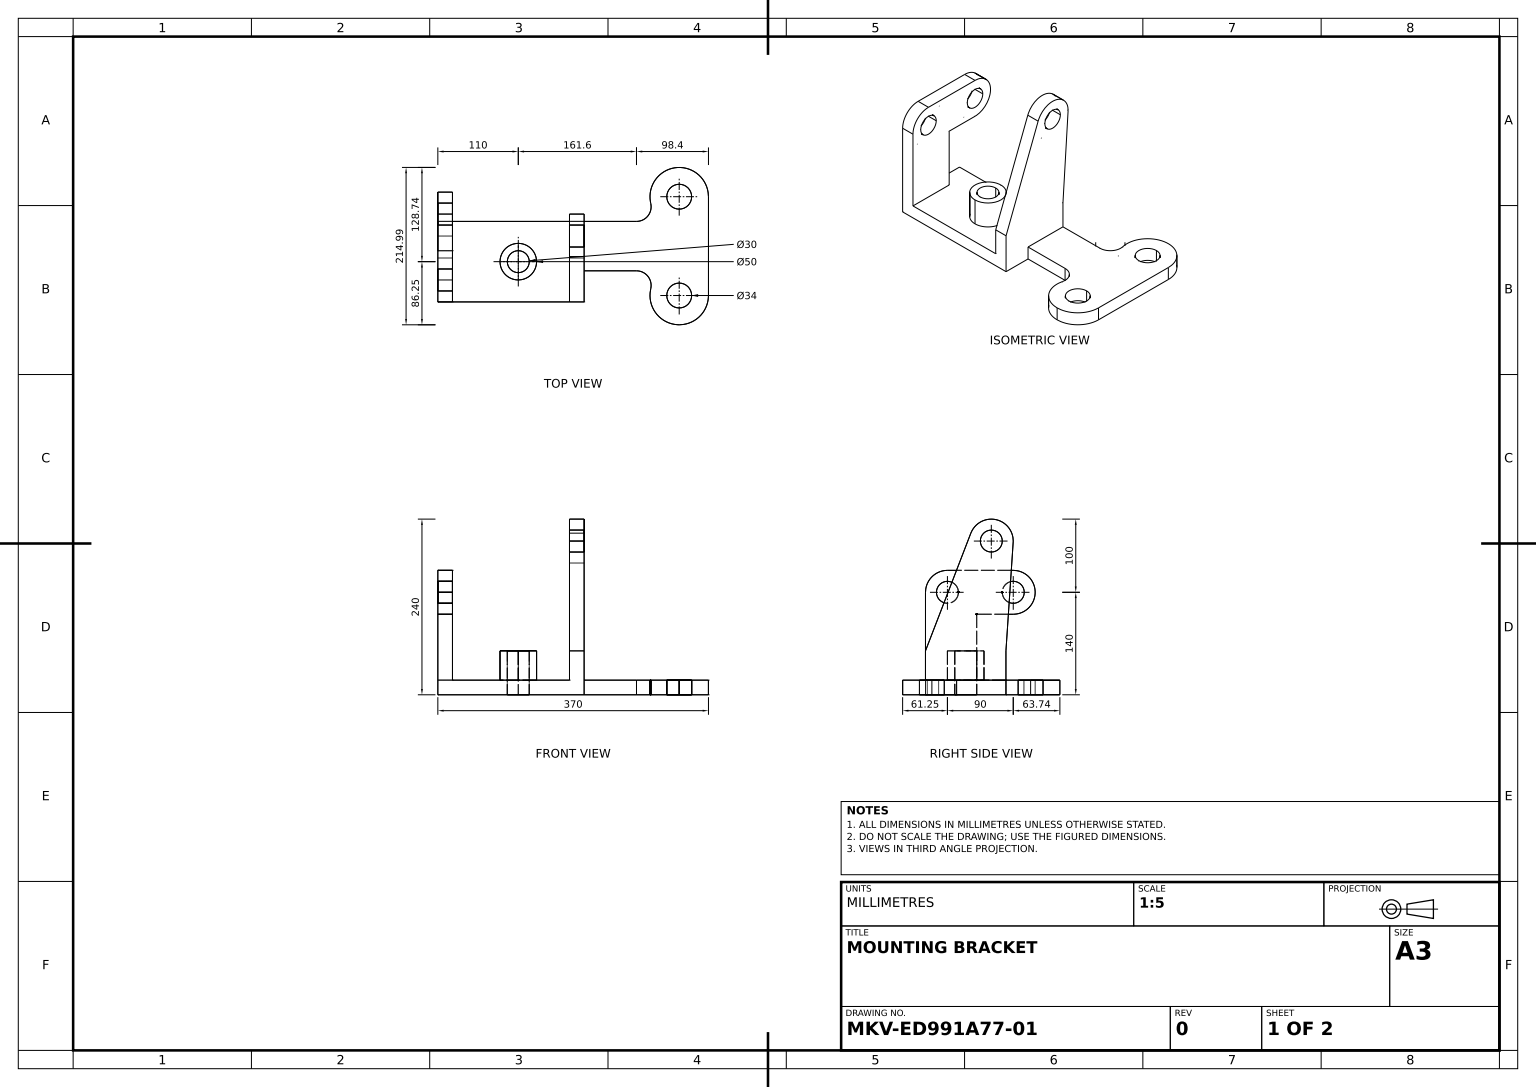
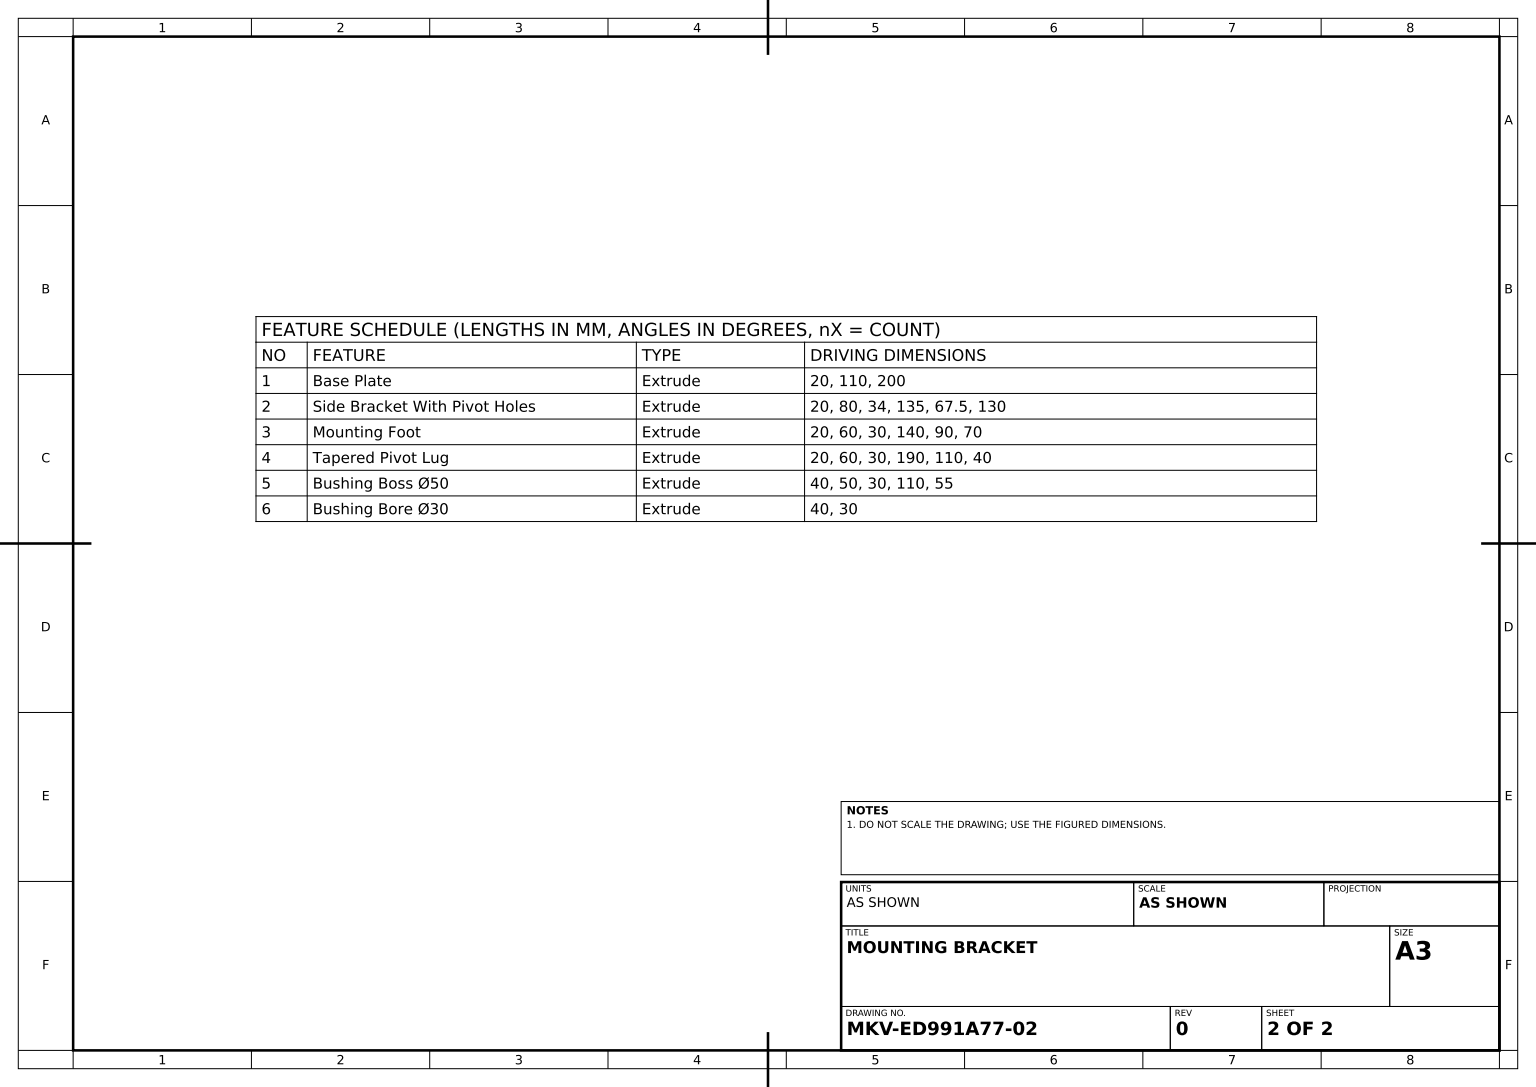
SolidWorks part; units mm, degrees
material "Plain Carbon Steel"
ref_plane "Front Plane" through (0, 0, 0) normal (0, 0, 1) x (1, 0, 0)
ref_plane "Top Plane" through (0, 0, 0) normal (0, 1, 0) x (1, 0, 0)
ref_plane "Right Plane" through (0, 0, 0) normal (1, 0, 0) x (0, 0, -1)
sketch "Base Plate Sketch" plane through (0, 0, 0) normal (0, 1, 0) x (1, 0, 0)
  line L1 (-100, 55) -> (100, 55)
  line L2 (-100, 55) -> (-100, -55)
  line L3 (-100, -55) -> (100, -55)
  line L4 (100, 55) -> (100, -55)
  line L5 (-100, 55) -> (100, -55) construction
  line L6 (-100, -55) -> (100, 55) construction
  point P0 (0, 0)
  dimension "D1" = 110
  dimension "D2" = 200
extrude "Base Plate" add sketch "Base Plate Sketch" along normal blind 20
sketch "Side Bracket Sketch" plane through (0, 20, 0) normal (0, 1, 0) x (1, 0, 0)
  line L0 (100, 55) -> (100, -12.5)
  line L1 (100, -55) -> (100, 55) construction
  line L2 (100, 55) -> (171.5968, 55)
  line L3 (100, -12.5) -> (171.5968, -12.5)
  line L4 (270, 88.75) -> (270, -46.25)
  circle A0 centre (230, 88.75) radius 17
  arc A1 (270, 88.75) -> (191.0645, 79.5833) centre (230, 88.75) ccw
  circle A2 centre (230, -46.25) radius 17
  arc A3 (191.0645, -37.0833) -> (270, -46.25) centre (230, -46.25) ccw
  arc A4 (171.5968, -12.5) -> (191.0645, -37.0833) centre (171.5968, -32.5) cw
  arc A5 (171.5968, 55) -> (191.0645, 79.5833) centre (171.5968, 75) ccw
  point P11 (100, 21.25)
  dimension "D1" = 80
  dimension "D2" = 34
  dimension "D3" = 80
  dimension "D4" = 34
  dimension "D9" = 20
  dimension "D5" = 135
  dimension "D6" = 67.5
  dimension "D7" = 67.5
  dimension "D8" = 130
  dimension "D10" = 67.5
  dimension "D11" = 135
extrude "Side Bracket With Pivot Holes" add sketch "Side Bracket Sketch" against normal blind 20
sketch "Mounting Foot Sketch" plane through (-100, 0, 0) normal (-1, 0, 0) x (0, 0, 1)
  line L0 (-65, 170) -> (25, 170)
  line L1 (-55, 0) -> (55, 0) construction
  line L2 (-15, 0) -> (55, 0)
  line L3 (55, 140) -> (55, 0)
  line L4 (55, 0) -> (-15, 0)
  line L5 (-65, 110) -> (-15, 110)
  line L6 (-15, 110) -> (-15, 0)
  circle A0 centre (25, 140) radius 15
  arc A1 (55, 140) -> (25, 170) centre (25, 140) ccw
  circle A2 centre (-65, 140) radius 15
  arc A3 (-65, 170) -> (-65, 110) centre (-65, 140) ccw
  line M4 (-55, 0) -> (55, 0)
  line M5 (55, 0) -> (55, 20)
  line M6 (55, 20) -> (-55, 20)
  dimension "D1" = 60
  dimension "D2" = 30
  dimension "D3" = 60
  dimension "D4" = 30
  dimension "D5" = 30
  dimension "D6" = 140
  dimension "D7" = 140
  dimension "D8" = 90
  dimension "D9" = 90
  dimension "D10" = 70
extrude "Mounting Foot" add sketch "Mounting Foot Sketch" against normal blind 20 contours L0 A3 L5 L6 L3 A1 A0 A2 M6 | L6 M6 M4 M5
sketch "Tapered Lug Sketch" plane through (100, 0, 0) normal (1, 0, 0) x (0, 0, -1)
  line L0 (-55, 20) -> (-55, 60)
  line L1 (-55, 20) -> (55, 20)
  line L2 (55, 20) -> (55, 60)
  line L3 (55, 60) -> (65, 210)
  line L4 (-55, 60) -> (7.0093, 220.7944)
  circle A0 centre (35, 210) radius 15
  arc A1 (64.7345, 206.0177) -> (7.0093, 220.7944) centre (35, 210) ccw
  line M7 (-12.5, 20) -> (-55, 20)
  dimension "D1" = 60
  dimension "D2" = 30
  dimension "D3" = 20
  dimension "D4" = 190
  dimension "D5" = 110
  dimension "D6" = 40
  dimension "D7" = 40
extrude "Tapered Pivot Lug" add sketch "Tapered Lug Sketch" against normal blind 20 contours L3 A1 L4 L0 L1 L2 A0 M7
sketch "Bushing Boss Sketch" plane through (0, 20, 0) normal (0, 1, 0) x (1, 0, 0)
  line L0 (-100, -25) -> (-100, -55) construction
  line L2 (-80, -55) -> (80, -55) construction
  circle A0 centre (10, 0) radius 15
  circle A1 centre (10, 0) radius 25
  dimension "D1" = 50
  dimension "D2" = 30
  dimension "D3" = 110
  dimension "D4" = 55
extrude "Bushing Boss Ø50" add sketch "Bushing Boss Sketch" along normal blind 40
sketch "Bushing Bore Sketch" plane through (0, 20, 0) normal (0, 1, 0) x (1, 0, 0)
  circle A0 centre (10, 0) radius 15
  dimension "D1" = 30
extrude "Bushing Bore Ø30" cut sketch "Bushing Bore Sketch" against normal blind 40
